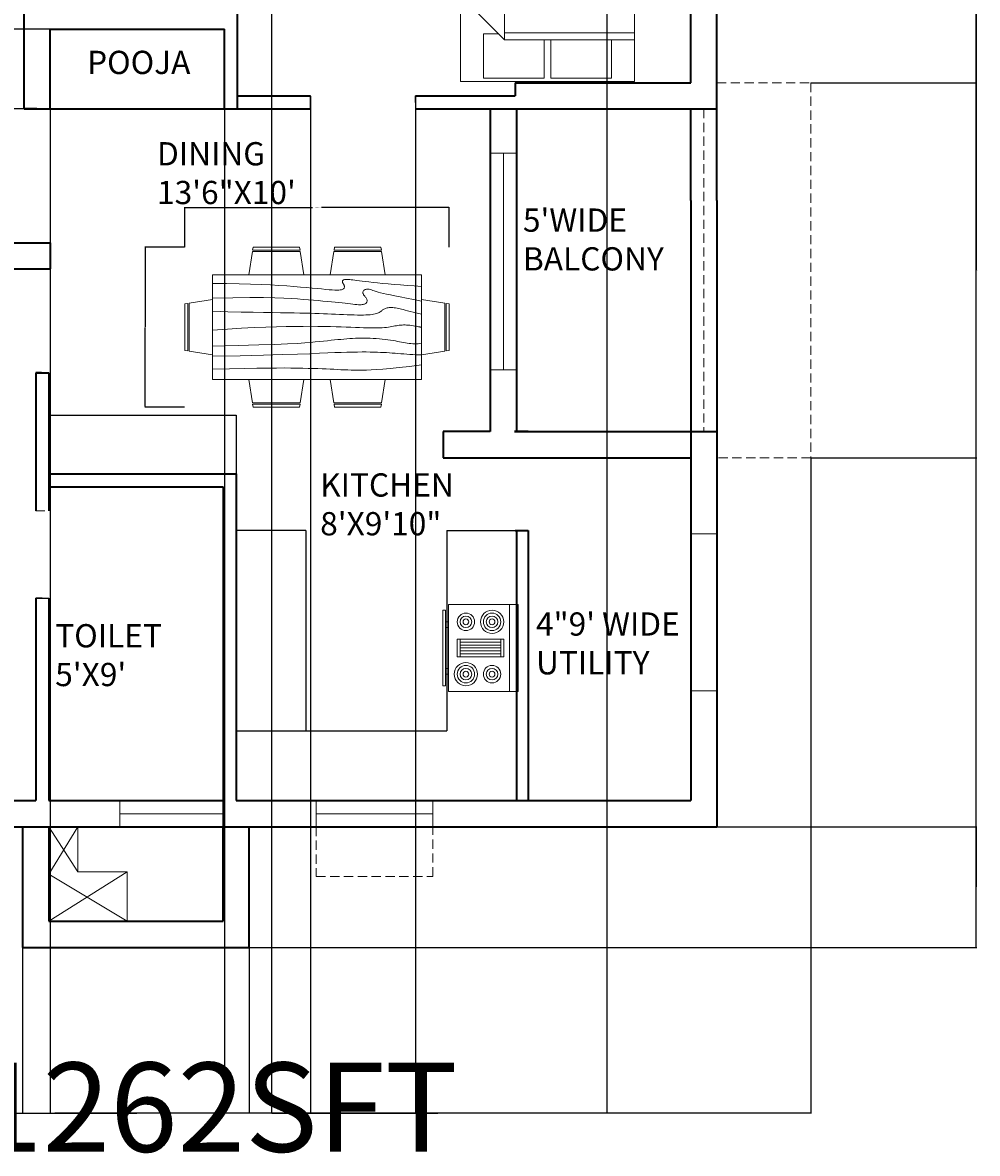
# Model space of a CAD drawing. Units: inches. Extents: x 276 to 912, y -567 to 621.
# Tile 3 of 7: x 583 to 912, y -567 to -178. Entities that reach past the tile are written whole.
import ezdxf

# ---------------------------------------------------------------- set-up
doc = ezdxf.new("R2010")
doc.units = ezdxf.units.IN
doc.linetypes.add('HIDDEN2', pattern=[4.7625, 3.175, -1.5875])
for name, color, linetype, lineweight in [('A-ANNO-DIMS', 2, 'Continuous', 18), ('A-ANNO-TEXT', 7, 'Continuous', 35), ('A-AREA-IDEN', 7, 'Continuous', 18), ('A-DOOR', 3, 'Continuous', 25), ('A-DOOR-HIDN', 3, 'HIDDEN2', 18), ('A-EQPM', 9, 'Continuous', 18), ('A-FLOR-CASE', 9, 'Continuous', 25), ('A-FLOR-OVHD', 8, 'HIDDEN2', 13), ('A-FLOR-SHFT', 8, 'Continuous', 18), ('A-FURN', 8, 'Continuous', 18), ('A-GLAZ', 4, 'Continuous', 18), ('A-WALL', 7, 'Continuous', 35), ('A-WALL-HIDN', 8, 'HIDDEN2', 18)]:
    doc.layers.add(name, color=color, linetype=linetype, lineweight=lineweight)
doc.dimstyles.get("Standard").update_dxf_attribs({"dimtxt": 0.18, "dimasz": 0.18, "dimexe": 0.18, "dimexo": 0.0625, "dimgap": 0.09, "dimtad": 0, "dimtih": 1, "dimtoh": 1, "dimdec": 4, "dimzin": 0, "dimdsep": 46, "dimtxsty": 'Standard', "dimcen": 0.09, "dimadec": 0, "dimazin": 0, "dimtfac": 1, "dimtdec": 4, "dimtofl": 0, "dimtmove": 0, "dimatfit": 3, "dimfxl": 1, "dimtolj": 1, "dimtzin": 0, "dimarcsym": 0})

# ---------------------------------------------------------------- blocks, each defined once
blk = doc.blocks.new('Dining Set - 36 x 72 in.')
for p, q in [((-22, 27.5), (-22.1562, 26.50042)), ((-22, 27.5), (-6, 27.5)), ((-5.8437, 26.49966), (-6, 27.5)), ((6, 27.5), (5.8438, 26.50042)), ((6, 27.5), (22, 27.5)), ((22.1563, 26.49966), (22, 27.5)), ((-22.2343, 26.00059), (-23.4847, 17.99762)), ((-22.2304, 26), (-5.7608, 26)), ((-5.8416, 26.5), (-22.1534, 26.5)), ((-4.5152, 17.99762), (-5.7655, 25.99926)), ((5.7657, 26.00059), (4.5153, 17.99762)), ((5.7696, 26), (22.2392, 26)), ((22.1584, 26.5), (5.8466, 26.5)), ((23.4848, 17.99762), (22.2345, 25.99926)), ((36, 18), (-36, 18)), ((-36, 18), (-36, -18)), ((36, -18), (36, 18)), ((-45.5, 8), (-44.5004, 8.15617)), ((-45.5, 8), (-45.5, -8)), ((-44.5, -8.15843), (-44.5, 8.15338)), ((-44.0006, 8.23428), (-35.9976, 9.48474)), ((-44, 8.23041), (-44, -8.23915)), ((44.0006, 8.23428), (35.9976, 9.48474)), ((44, 8.23041), (44, -8.23915)), ((44.5, -8.15843), (44.5, 8.15338)), ((45.5, 8), (44.5005, 8.15617)), ((45.5, 8), (45.5, -8)), ((-44.4997, -8.15631), (-45.5, -8)), ((-35.9976, -9.48476), (-43.9993, -8.2345)), ((35.9976, -9.48476), (43.9993, -8.2345)), ((44.4997, -8.15631), (45.5, -8)), ((-36, -18), (36, -18)), ((-22.2343, -26.0006), (-23.4847, -17.99762)), ((-4.5152, -17.99762), (-5.7655, -25.99928)), ((5.7657, -26.0006), (4.5153, -17.99762)), ((23.4848, -17.99762), (22.2345, -25.99928)), ((-22.2304, -26), (-5.7608, -26)), ((-22, -27.5), (-22.1562, -26.50044)), ((-5.8416, -26.5), (-22.1534, -26.5)), ((-5.8437, -26.49967), (-6, -27.5)), ((5.7696, -26), (22.2392, -26)), ((6, -27.5), (5.8438, -26.50044)), ((22.1584, -26.5), (5.8466, -26.5)), ((22.1563, -26.49967), (22, -27.5)), ((-22, -27.5), (-6, -27.5)), ((6, -27.5), (22, -27.5))]:
    blk.add_line(p, q)
for points in [[(-36, 15), (-31.1772, 14.97754), (-26.8079, 14.91406), (-22.8538, 14.81543), (-19.276, 14.6875), (-16.0362, 14.53613), (-13.0957, 14.36718), (-10.4159, 14.18652), (-7.9583, 14), (-5.6904, 13.81315), (-3.6035, 13.63021), (-1.6954, 13.45508), (0.0365, 13.29166), (1.5945, 13.14388), (2.9811, 13.01562), (4.1988, 12.9108), (5.25, 12.83333), (6.1393, 12.78613), (6.8802, 12.76823), (7.4883, 12.77767), (7.9792, 12.8125), (8.3685, 12.87077), (8.6719, 12.95052), (8.9049, 13.0498), (9.0833, 13.16666), (9.2205, 13.29899), (9.3216, 13.44401), (9.3895, 13.59879), (9.4271, 13.76041), (9.4373, 13.92594), (9.4232, 14.09245), (9.3875, 14.257), (9.3333, 14.41666), (9.2638, 14.56917), (9.1836, 14.71484), (9.0975, 14.85465), (9.0104, 14.98958), (8.9272, 15.1206), (8.8529, 15.2487), (8.7922, 15.37483), (8.75, 15.5), (8.7305, 15.62467), (8.7344, 15.74739), (8.7617, 15.86621), (8.8125, 15.97916), (8.8867, 16.08431), (8.9844, 16.17968), (9.1055, 16.26334), (9.25, 16.33333), (9.4189, 16.38802), (9.6172, 16.42708), (9.8506, 16.45052), (10.125, 16.45833), (10.4463, 16.45052), (10.8203, 16.42708), (11.2529, 16.38802), (11.75, 16.33333), (12.3184, 16.26318), (12.9694, 16.17838), (13.7151, 16.07991), (14.5677, 15.96875), (15.5395, 15.84586), (16.6426, 15.71224), (17.8893, 15.56884), (19.2917, 15.41666), (20.859, 15.25667), (22.5879, 15.08984), (24.4721, 14.91715), (26.5052, 14.73958), (28.6809, 14.5581), (30.9929, 14.3737), (33.4347, 14.18733), (36, 14)], [(-36, 10), (-28.9766, 10.14274), (-23.1725, 10.20442), (-18.4241, 10.19775), (-14.5677, 10.13541), (-11.4399, 10.03011), (-8.877, 9.89453), (-6.7154, 9.74137), (-4.7917, 9.58333), (-2.9698, 9.43082), (-1.2246, 9.28515), (0.4415, 9.14534), (2.026, 9.01041), (3.5266, 8.87939), (4.9408, 8.7513), (6.266, 8.62516), (7.5, 8.5), (8.6411, 8.37549), (9.6914, 8.2539), (10.6538, 8.13818), (11.5312, 8.03125), (12.3267, 7.93603), (13.043, 7.85547), (13.6831, 7.79248), (14.25, 7.75), (14.7471, 7.7303), (15.1797, 7.73307), (15.5537, 7.75732), (15.875, 7.80208), (16.1494, 7.86637), (16.3828, 7.94922), (16.5811, 8.04964), (16.75, 8.16666), (16.8944, 8.29915), (17.0143, 8.44531), (17.1089, 8.60319), (17.1771, 8.77083), (17.218, 8.94629), (17.2305, 9.1276), (17.2137, 9.31282), (17.1667, 9.5), (17.0895, 9.6875), (16.987, 9.875), (16.8649, 10.0625), (16.7292, 10.25), (16.5856, 10.4375), (16.4401, 10.625), (16.2985, 10.8125), (16.1667, 11), (16.05, 11.18733), (15.9518, 11.3737), (15.8752, 11.5581), (15.8229, 11.73958), (15.798, 11.91715), (15.8034, 12.08984), (15.842, 12.25667), (15.9167, 12.41666), (16.0295, 12.56836), (16.1784, 12.70833), (16.3605, 12.83268), (16.5729, 12.9375), (16.8127, 13.01888), (17.0768, 13.07291), (17.3625, 13.0957), (17.6667, 13.08333), (17.9894, 13.03312), (18.3418, 12.94726), (18.7382, 12.82918), (19.1927, 12.68229), (19.7195, 12.51001), (20.3327, 12.31575), (21.0465, 12.10294), (21.875, 11.875), (22.8357, 11.63354), (23.959, 11.37304), (25.2786, 11.08618), (26.8282, 10.76562), (28.6414, 10.40405), (30.752, 9.99414), (33.1936, 9.52856), (36, 9)], [(-36, 5.5), (-30.7157, 5.3348), (-26.069, 5.20963), (-21.9946, 5.11767), (-18.4271, 5.05208), (-15.3009, 5.00602), (-12.5508, 4.97265), (-10.1112, 4.94515), (-7.9167, 4.91666), (-5.909, 4.88167), (-4.0586, 4.83984), (-2.3429, 4.79215), (-0.7396, 4.73958), (0.7739, 4.6831), (2.22, 4.6237), (3.6213, 4.56233), (5, 4.5), (6.373, 4.43782), (7.7344, 4.3776), (9.0723, 4.32129), (10.375, 4.27083), (11.6309, 4.22819), (12.8281, 4.19531), (13.9551, 4.17415), (15, 4.16666), (15.954, 4.17448), (16.819, 4.19791), (17.6001, 4.23698), (18.3021, 4.29166), (18.9299, 4.36198), (19.4883, 4.44791), (19.9823, 4.54948), (20.4167, 4.66666), (20.7969, 4.79899), (21.1302, 4.94401), (21.4245, 5.09879), (21.6875, 5.26041), (21.9271, 5.42594), (22.1511, 5.59245), (22.3672, 5.757), (22.5834, 5.91666), (22.8065, 6.06868), (23.0404, 6.21093), (23.2879, 6.34147), (23.5521, 6.45833), (23.8358, 6.55957), (24.142, 6.64323), (24.4735, 6.70735), (24.8334, 6.75), (25.2235, 6.76969), (25.642, 6.76692), (26.0858, 6.74267), (26.5521, 6.69791), (27.0379, 6.63362), (27.5404, 6.55078), (28.0565, 6.45036), (28.5834, 6.33333), (29.1242, 6.19987), (29.7071, 6.04687), (30.3661, 5.87044), (31.1354, 5.66666), (32.0493, 5.43164), (33.142, 5.16146), (34.4475, 4.85221), (36, 4.5)], [(-36, -1), (-30.7915, -0.6591), (-26.0195, -0.38216), (-21.6519, -0.16284), (-17.6563, 0.00521), (-14.0005, 0.12833), (-10.6523, 0.21289), (-7.5796, 0.26522), (-4.75, 0.29166), (-2.134, 0.29793), (0.2878, 0.28711), (2.5317, 0.26163), (4.6146, 0.22396), (6.5529, 0.17651), (8.3633, 0.12174), (10.0623, 0.06209), (11.6667, 0), (13.1899, -0.06201), (14.6341, -0.1211), (15.9982, -0.17432), (17.2813, -0.21875), (18.4823, -0.25147), (19.6003, -0.26953), (20.6343, -0.27002), (21.5834, -0.25), (22.4481, -0.20768), (23.2357, -0.14584), (23.9549, -0.06836), (24.6146, 0.02083), (25.2235, 0.11784), (25.7904, 0.21875), (26.3241, 0.31966), (26.8334, 0.41666), (27.3265, 0.50618), (27.8099, 0.58593), (28.2894, 0.65397), (28.7709, 0.70833), (29.2601, 0.74707), (29.763, 0.76823), (30.2855, 0.76985), (30.8334, 0.75), (31.4088, 0.70784), (31.9994, 0.64713), (32.589, 0.57275), (33.1615, 0.48958), (33.7008, 0.4025), (34.1908, 0.3164), (34.6153, 0.23616), (34.9584, 0.16666), (35.2099, 0.11165), (35.3848, 0.07031), (35.504, 0.04069), (35.5886, 0.02083), (35.6594, 0.00879), (35.7377, 0.0026), (35.8442, 0.00032), (36, 0)], [(-36, -6.5), (-27.1843, -6.31267), (-20.084, -6.1263), (-14.469, -5.9419), (-10.1094, -5.76042), (-6.7752, -5.58285), (-4.2363, -5.41016), (-2.2629, -5.24333), (-0.625, -5.08334), (0.8708, -4.93099), (2.2715, -4.78646), (3.5872, -4.64974), (4.8281, -4.52084), (6.0046, -4.39974), (7.127, -4.28646), (8.2053, -4.18099), (9.25, -4.08334), (10.2705, -3.99382), (11.2734, -3.91407), (12.2647, -3.84603), (13.25, -3.79167), (14.2354, -3.75293), (15.2266, -3.73177), (16.2295, -3.73015), (17.25, -3.75), (18.2912, -3.79248), (19.3451, -3.85547), (20.4009, -3.93604), (21.4479, -4.03125), (22.4754, -4.13819), (23.4727, -4.25391), (24.4289, -4.37549), (25.3334, -4.5), (26.1785, -4.62492), (26.9694, -4.74935), (27.7145, -4.87281), (28.4219, -4.99479), (29.1, -5.11483), (29.7572, -5.23242), (30.4016, -5.34709), (31.0417, -5.45834), (31.6837, -5.56437), (32.3262, -5.65821), (32.9658, -5.73153), (33.599, -5.77604), (34.2224, -5.78345), (34.8327, -5.74545), (35.4264, -5.65373), (36, -5.5)], [(-36, -10), (-26.4022, -9.81299), (-18.4675, -9.62891), (-11.9839, -9.45069), (-6.7396, -9.28125), (-2.5226, -9.12354), (0.8789, -8.98047), (3.6769, -8.85498), (6.0833, -8.75), (8.2767, -8.66765), (10.3021, -8.60677), (12.1712, -8.56543), (13.8958, -8.54167), (15.4876, -8.53353), (16.9583, -8.53907), (18.3197, -8.55632), (19.5834, -8.58334), (20.7616, -8.61841), (21.8685, -8.66081), (22.9188, -8.71004), (23.9271, -8.76563), (24.9081, -8.82707), (25.8763, -8.89388), (26.8465, -8.96558), (27.8334, -9.04167), (28.8474, -9.12118), (29.8828, -9.20117), (30.93, -9.27824), (31.9792, -9.34896), (33.0205, -9.40991), (34.0443, -9.45768), (35.0407, -9.48885), (36, -9.5)], [(-36, -14.5), (-30.0881, -14.33513), (-25.0332, -14.21224), (-20.7312, -14.12647), (-17.0781, -14.07292), (-13.97, -14.04671), (-11.3027, -14.04297), (-8.9724, -14.05681), (-6.875, -14.08334), (-4.9224, -14.11833), (-3.0905, -14.16016), (-1.3709, -14.20785), (0.2448, -14.26042), (1.7647, -14.3169), (3.1973, -14.3763), (4.5507, -14.43767), (5.8333, -14.5), (7.0554, -14.5621), (8.235, -14.62175), (9.3922, -14.67652), (10.5469, -14.72396), (11.7192, -14.76164), (12.929, -14.78711), (14.1965, -14.79794), (15.5417, -14.79167), (16.9933, -14.76424), (18.6152, -14.70508), (20.4804, -14.60197), (22.6615, -14.44271), (25.2312, -14.21509), (28.2624, -13.9069), (31.8277, -13.50594), (36, -13)]]:
    blk.add_lwpolyline(points)
blk = doc.blocks.new('Bed - Queen')
for p, q in [((0, -80.00003), (0, 0)), ((0, 0), (59.99999, 0)), ((59.99999, 0), (59.99999, -80.00003)), ((7.99999, -1.2), (28.79998, -1.2)), ((7.99999, -14.4), (7.99999, -1.2)), ((28.79998, -1.2), (28.79998, -14.4)), ((31.19999, -1.2), (51.99999, -1.2)), ((31.19999, -14.4), (31.19999, -1.2)), ((51.99999, -1.2), (51.99999, -16.4)), ((0, -14.4), (44.8, -14.4)), ((59.99999, -29.6), (44.8, -14.4)), ((44.8, -14.4), (44.8, -29.6)), ((44.8, -16.8), (0, -16.8)), ((51.99999, -16.4), (46.79936, -16.4)), ((44.8, -29.6), (59.99999, -29.6)), ((59.99999, -80.00003), (0, -80.00003))]:
    blk.add_line(p, q)
blk = doc.blocks.new('Range-Oven - 30 in top')
for p, q in [((0, -3), (30, -3)), ((12, -6), (18, -6)), ((13, -20), (13, -6)), ((14, -6), (14, -20)), ((15, -20), (15, -6)), ((16, -6), (16, -20)), ((17, -20), (17, -6)), ((18, -20), (12, -20)), ((6, -24), (6, -25)), ((8, -25), (8, -24)), ((22, -25), (22, -24)), ((24, -24), (24, -25))]:
    blk.add_line(p, q)
for points in [[(0, -24), (0, 0), (30, 0), (30, -24)], [(12, -21), (12, -5), (18, -5), (18, -21)], [(2, -26), (2, -25), (28, -25), (28, -26)]]:
    blk.add_lwpolyline(points, close=True)
for centre, radius in [((6, -9), 4), ((6, -9), 3), ((6, -9), 2), ((24, -9), 3), ((24, -9), 2), ((6, -9), 1), ((24, -9), 1), ((6, -18), 3), ((24, -18), 4), ((24, -18), 3), ((6, -18), 2), ((6, -18), 1), ((24, -18), 2), ((24, -18), 1)]:
    blk.add_circle(centre, radius)
blk = doc.blocks.new('DOOR-JAMB-4.5IN')
for p, q in [((0, 2.25), (0, 4.5)), ((0, 4.5), (0, 0))]:
    blk.add_line(p, q)
blk = doc.blocks.new('*D18')
at = {"layer": 'A-ANNO-DIMS', "color": 0, "lineweight": -2, "transparency": 16777216}
for p, q in [((638.77, -255.04), (638.77, -241.28)), ((638.95, -241.46), (682.74, -241.46)), ((729.59, -241.46), (685.8, -241.46)), ((729.77, -255.04), (729.77, -241.28))]:
    blk.add_line(p, q, dxfattribs=at)
at = {"layer": 'A-ANNO-DIMS', "color": 0, "transparency": 16777216}
for points in [[(638.95, -241.43), (638.95, -241.49), (638.77, -241.46)], [(729.59, -241.43), (729.59, -241.49), (729.77, -241.46)]]:
    blk.add_solid(points, dxfattribs=at)
at = {"layer": 'Defpoints', "color": 0, "transparency": 16777216}
for p in [(729.77, -241.46), (638.77, -255.11), (729.77, -255.11)]:
    blk.add_point(p, dxfattribs=at)
at = {"layer": 'A-ANNO-DIMS', "color": 0, "transparency": 16777216, "insert": (684.27, -241.46), "char_height": 0.18, "attachment_point": 5}
blk.add_mtext('\\A1;DINING SET 91 TYP.', dxfattribs=at)
blk = doc.blocks.new('*D19')
at = {"layer": 'A-ANNO-DIMS', "color": 0, "lineweight": -2, "transparency": 16777216}
for p, q in [((638.7, -255.11), (624.94, -255.11)), ((625.12, -255.29), (625.12, -282.43)), ((625.12, -309.93), (625.12, -282.79)), ((638.7, -310.11), (624.94, -310.11))]:
    blk.add_line(p, q, dxfattribs=at)
at = {"layer": 'A-ANNO-DIMS', "color": 0, "transparency": 16777216}
for points in [[(625.09, -255.29), (625.15, -255.29), (625.12, -255.11)], [(625.09, -309.93), (625.15, -309.93), (625.12, -310.11)]]:
    blk.add_solid(points, dxfattribs=at)
at = {"layer": 'Defpoints', "color": 0, "transparency": 16777216}
for p in [(625.12, -255.11), (638.77, -255.11), (638.77, -310.11)]:
    blk.add_point(p, dxfattribs=at)
at = {"layer": 'A-ANNO-DIMS', "color": 0, "transparency": 16777216, "insert": (625.12, -282.61), "char_height": 0.18, "attachment_point": 5}
blk.add_mtext('\\A1;55 TYP.', dxfattribs=at)
blk = doc.blocks.new('*D24')
at = {"layer": 'A-ANNO-DIMS', "color": 0, "lineweight": -2, "transparency": 16777216}
for p, q in [((333.082179, 103.255751), (333.082179, -553.223061)), ((854.209085, -327.604004), (854.209085, -553.223061)), ((333.262179, -553.043061), (593.255632, -553.043061)), ((854.029085, -553.043061), (594.035632, -553.043061))]:
    blk.add_line(p, q, dxfattribs=at)
at = {"layer": 'A-ANNO-DIMS', "color": 0, "transparency": 16777216}
for points in [[(333.262179, -553.013061), (333.262179, -553.073061), (333.082179, -553.043061)], [(854.029085, -553.013061), (854.029085, -553.073061), (854.209085, -553.043061)]]:
    blk.add_solid(points, dxfattribs=at)
at = {"layer": 'Defpoints', "color": 0, "transparency": 16777216}
for p in [(333.082179, 103.318251), (854.209085, -327.541504), (854.209085, -553.043061)]:
    blk.add_point(p, dxfattribs=at)
at = {"layer": 'A-ANNO-DIMS', "color": 0, "transparency": 16777216, "insert": (593.645632, -553.043061), "char_height": 0.18, "attachment_point": 5}
blk.add_mtext('\\A1;521.1', dxfattribs=at)
blk = doc.blocks.new('*D25')
at = {"layer": 'A-ANNO-DIMS', "color": 0, "lineweight": -2, "transparency": 16777216}
for p, q in [((478.5, 564.29), (911.39, 564.29)), ((911.21, 564.11), (911.21, 34.31)), ((911.21, -495.86), (911.21, 33.95)), ((582.98, -496.04), (911.39, -496.04))]:
    blk.add_line(p, q, dxfattribs=at)
at = {"layer": 'A-ANNO-DIMS', "color": 0, "transparency": 16777216}
for points in [[(911.18, 564.11), (911.24, 564.11), (911.21, 564.29)], [(911.18, -495.86), (911.24, -495.86), (911.21, -496.04)]]:
    blk.add_solid(points, dxfattribs=at)
at = {"layer": 'Defpoints', "color": 0, "transparency": 16777216}
for p in [(478.44, 564.29), (582.92, -496.04), (911.21, -496.04)]:
    blk.add_point(p, dxfattribs=at)
at = {"layer": 'A-ANNO-DIMS', "color": 0, "transparency": 16777216, "insert": (911.21, 34.13), "char_height": 0.18, "attachment_point": 5}
blk.add_mtext('\\A1;1060.3', dxfattribs=at)
blk = doc.blocks.new('*D33')
at = {"layer": 'A-ANNO-DIMS', "color": 0, "lineweight": -2, "transparency": 16777216}
for p, q in [((553.582179, 65.246155), (553.582179, -553.223061)), ((668.582179, 65.246155), (668.582179, -553.223061)), ((553.762179, -553.043061), (610.812179, -553.043061)), ((668.402179, -553.043061), (611.352179, -553.043061))]:
    blk.add_line(p, q, dxfattribs=at)
at = {"layer": 'A-ANNO-DIMS', "color": 0, "transparency": 16777216}
for points in [[(553.762179, -553.013061), (553.762179, -553.073061), (553.582179, -553.043061)], [(668.402179, -553.013061), (668.402179, -553.073061), (668.582179, -553.043061)]]:
    blk.add_solid(points, dxfattribs=at)
at = {"layer": 'Defpoints', "color": 0, "transparency": 16777216}
for p in [(553.582179, 65.308655), (668.582179, 65.308655), (668.582179, -553.043061)]:
    blk.add_point(p, dxfattribs=at)
at = {"layer": 'A-ANNO-DIMS', "color": 0, "transparency": 16777216, "insert": (611.082179, -553.043061), "char_height": 0.18, "attachment_point": 5}
blk.add_mtext('\\A1;115', dxfattribs=at)
blk = doc.blocks.new('*D34')
at = {"layer": 'A-ANNO-DIMS', "color": 0, "lineweight": -2, "transparency": 16777216}
for p, q in [((668.58, 65.25), (668.58, -553.22)), ((784, 65.25), (784, -553.22)), ((668.76, -553.04), (725.81, -553.04)), ((783.82, -553.04), (726.77, -553.04))]:
    blk.add_line(p, q, dxfattribs=at)
at = {"layer": 'A-ANNO-DIMS', "color": 0, "transparency": 16777216}
for points in [[(668.76, -553.01), (668.76, -553.07), (668.58, -553.04)], [(783.82, -553.01), (783.82, -553.07), (784, -553.04)]]:
    blk.add_solid(points, dxfattribs=at)
at = {"layer": 'Defpoints', "color": 0, "transparency": 16777216}
for p in [(668.58, 65.31), (784, 65.31), (784, -553.04)]:
    blk.add_point(p, dxfattribs=at)
at = {"layer": 'A-ANNO-DIMS', "color": 0, "transparency": 16777216, "insert": (726.29, -553.04), "char_height": 0.18, "attachment_point": 5}
blk.add_mtext('\\A1;115.42', dxfattribs=at)
blk = doc.blocks.new('*D54')
at = {"layer": 'A-ANNO-DIMS', "color": 0, "lineweight": -2, "transparency": 16777216}
for p, q in [((821.980989, -64.541504), (911.389085, -64.541504)), ((911.209085, -64.721504), (911.209085, -259.361504)), ((911.209085, -454.361504), (911.209085, -259.721504)), ((821.980989, -454.541504), (911.389085, -454.541504))]:
    blk.add_line(p, q, dxfattribs=at)
at = {"layer": 'A-ANNO-DIMS', "color": 0, "transparency": 16777216}
for points in [[(911.179085, -64.721504), (911.239085, -64.721504), (911.209085, -64.541504)], [(911.179085, -454.361504), (911.239085, -454.361504), (911.209085, -454.541504)]]:
    blk.add_solid(points, dxfattribs=at)
at = {"layer": 'Defpoints', "color": 0, "transparency": 16777216}
for p in [(821.918489, -64.541504), (821.918489, -454.541504), (911.209085, -454.541504)]:
    blk.add_point(p, dxfattribs=at)
at = {"layer": 'A-ANNO-DIMS', "color": 0, "transparency": 16777216, "insert": (911.209085, -259.541504), "char_height": 0.18, "attachment_point": 5}
blk.add_mtext('\\A1;390', dxfattribs=at)
blk = doc.blocks.new('*D57')
at = {"layer": 'A-ANNO-DIMS', "color": 0, "lineweight": -2, "transparency": 16777216}
for p, q in [((582.918489, -496.105561), (582.918489, -553.223061)), ((660.918489, -496.105561), (660.918489, -553.223061)), ((583.098489, -553.043061), (621.678489, -553.043061)), ((660.738489, -553.043061), (622.158489, -553.043061))]:
    blk.add_line(p, q, dxfattribs=at)
at = {"layer": 'A-ANNO-DIMS', "color": 0, "transparency": 16777216}
for points in [[(583.098489, -553.013061), (583.098489, -553.073061), (582.918489, -553.043061)], [(660.738489, -553.013061), (660.738489, -553.073061), (660.918489, -553.043061)]]:
    blk.add_solid(points, dxfattribs=at)
at = {"layer": 'Defpoints', "color": 0, "transparency": 16777216}
for p in [(582.918489, -496.043061), (660.918489, -496.043061), (660.918489, -553.043061)]:
    blk.add_point(p, dxfattribs=at)
at = {"layer": 'A-ANNO-DIMS', "color": 0, "transparency": 16777216, "insert": (621.918489, -553.043061), "char_height": 0.18, "attachment_point": 5}
blk.add_mtext('\\A1;78', dxfattribs=at)
blk = doc.blocks.new('*D58')
at = {"layer": 'A-ANNO-DIMS', "color": 0, "lineweight": -2, "transparency": 16777216}
for p, q in [((660.98, -454.54), (911.39, -454.54)), ((911.21, -454.72), (911.21, -475.11)), ((911.21, -495.86), (911.21, -475.47)), ((660.98, -496.04), (911.39, -496.04))]:
    blk.add_line(p, q, dxfattribs=at)
at = {"layer": 'A-ANNO-DIMS', "color": 0, "transparency": 16777216}
for points in [[(911.18, -454.72), (911.24, -454.72), (911.21, -454.54)], [(911.18, -495.86), (911.24, -495.86), (911.21, -496.04)]]:
    blk.add_solid(points, dxfattribs=at)
at = {"layer": 'Defpoints', "color": 0, "transparency": 16777216}
for p in [(660.92, -454.54), (911.21, -454.54), (660.92, -496.04)]:
    blk.add_point(p, dxfattribs=at)
at = {"layer": 'A-ANNO-DIMS', "color": 0, "transparency": 16777216, "insert": (911.21, -475.29), "char_height": 0.18, "attachment_point": 5}
blk.add_mtext('\\A1;41.5', dxfattribs=at)
blk = doc.blocks.new('*D63')
at = {"layer": 'A-ANNO-DIMS', "color": 0, "lineweight": -2, "transparency": 16777216}
for p, q in [((682.059922, -203.068216), (682.059922, -553.223061)), ((718.16583, -207.568216), (718.16583, -553.223061)), ((682.239922, -553.043061), (699.617876, -553.043061)), ((717.98583, -553.043061), (700.607876, -553.043061))]:
    blk.add_line(p, q, dxfattribs=at)
at = {"layer": 'A-ANNO-DIMS', "color": 0, "transparency": 16777216}
for points in [[(682.239922, -553.013061), (682.239922, -553.073061), (682.059922, -553.043061)], [(717.98583, -553.013061), (717.98583, -553.073061), (718.16583, -553.043061)]]:
    blk.add_solid(points, dxfattribs=at)
at = {"layer": 'Defpoints', "color": 0, "transparency": 16777216}
for p in [(682.059922, -203.005716), (718.16583, -207.505716), (718.16583, -553.043061)]:
    blk.add_point(p, dxfattribs=at)
at = {"layer": 'A-ANNO-DIMS', "color": 0, "transparency": 16777216, "insert": (700.112876, -553.043061), "char_height": 0.18, "attachment_point": 5}
blk.add_mtext('\\A1;36.106', dxfattribs=at)
blk = doc.blocks.new('*D68')
at = {"layer": 'A-ANNO-DIMS', "color": 0, "lineweight": -2, "transparency": 16777216}
for p, q in [((592.418489, -207.568216), (592.418489, -553.223061)), ((652.418489, -207.568216), (652.418489, -553.223061)), ((592.598489, -553.043061), (622.193489, -553.043061)), ((652.238489, -553.043061), (622.643489, -553.043061))]:
    blk.add_line(p, q, dxfattribs=at)
at = {"layer": 'A-ANNO-DIMS', "color": 0, "transparency": 16777216}
for points in [[(592.598489, -553.013061), (592.598489, -553.073061), (592.418489, -553.043061)], [(652.238489, -553.013061), (652.238489, -553.073061), (652.418489, -553.043061)]]:
    blk.add_solid(points, dxfattribs=at)
at = {"layer": 'Defpoints', "color": 0, "transparency": 16777216}
for p in [(592.418489, -207.505716), (652.418489, -207.505716), (652.418489, -553.043061)]:
    blk.add_point(p, dxfattribs=at)
at = {"layer": 'A-ANNO-DIMS', "color": 0, "transparency": 16777216, "insert": (622.418489, -553.043061), "char_height": 0.18, "attachment_point": 5}
blk.add_mtext('\\A1;60', dxfattribs=at)
blk = doc.blocks.new('*D69')
at = {"layer": 'A-ANNO-DIMS', "color": 0, "lineweight": -2, "transparency": 16777216}
for p, q in [((592.355989, -180.041504), (275.902179, -180.041504)), ((276.082179, -180.221504), (276.082179, -193.59361)), ((276.082179, -207.325716), (276.082179, -193.95361)), ((592.355989, -207.505716), (275.902179, -207.505716))]:
    blk.add_line(p, q, dxfattribs=at)
at = {"layer": 'A-ANNO-DIMS', "color": 0, "transparency": 16777216}
for points in [[(276.052179, -180.221504), (276.112179, -180.221504), (276.082179, -180.041504)], [(276.052179, -207.325716), (276.112179, -207.325716), (276.082179, -207.505716)]]:
    blk.add_solid(points, dxfattribs=at)
at = {"layer": 'Defpoints', "color": 0, "transparency": 16777216}
for p in [(276.082179, -180.041504), (592.418489, -180.041504), (592.418489, -207.505716)]:
    blk.add_point(p, dxfattribs=at)
at = {"layer": 'A-ANNO-DIMS', "color": 0, "transparency": 16777216, "insert": (276.082179, -193.77361), "char_height": 0.18, "attachment_point": 5}
blk.add_mtext('\\A1;27.464', dxfattribs=at)
blk = doc.blocks.new('*D78')
at = {"layer": 'A-ANNO-DIMS', "color": 0, "lineweight": -2, "transparency": 16777216}
for p, q in [((854.271585, -198.505716), (911.389085, -198.505716)), ((911.209085, -198.685716), (911.209085, -262.84361)), ((911.209085, -327.361504), (911.209085, -263.20361)), ((854.271585, -327.541504), (911.389085, -327.541504))]:
    blk.add_line(p, q, dxfattribs=at)
at = {"layer": 'A-ANNO-DIMS', "color": 0, "transparency": 16777216}
for points in [[(911.179085, -198.685716), (911.239085, -198.685716), (911.209085, -198.505716)], [(911.179085, -327.361504), (911.239085, -327.361504), (911.209085, -327.541504)]]:
    blk.add_solid(points, dxfattribs=at)
at = {"layer": 'Defpoints', "color": 0, "transparency": 16777216}
for p in [(854.209085, -198.505716), (854.209085, -327.541504), (911.209085, -327.541504)]:
    blk.add_point(p, dxfattribs=at)
at = {"layer": 'A-ANNO-DIMS', "color": 0, "transparency": 16777216, "insert": (911.209085, -263.02361), "char_height": 0.18, "attachment_point": 5}
blk.add_mtext('\\A1;129.04', dxfattribs=at)

msp = doc.modelspace()

# ---------------------------------------------------------------- linework, layer by layer
at = {"layer": 'A-DOOR-HIDN'}
msp.add_line((587.4185, -345.8507), (591.9185, -345.8507), dxfattribs=at)
at = {"layer": 'A-FLOR-CASE'}
for p, q in [((591.9185, -312.8352), (656.4185, -312.8352)), ((656.4185, -312.8352), (656.4185, -333.0415)), ((680.4185, -352.5843), (656.4185, -352.5843)), ((680.4185, -352.5843), (680.4185, -421.5415)), ((728.9185, -352.5843), (728.9185, -421.5415)), ((728.9185, -352.5843), (752.4185, -352.5843)), ((656.4185, -421.5415), (728.9185, -421.5415))]:
    msp.add_line(p, q, dxfattribs=at)
at = {"layer": 'A-FLOR-OVHD'}
for p, q in [((821.9185, -198.5057), (854.2091, -198.5057)), ((854.2091, -198.5057), (854.2091, -327.5415)), ((854.2091, -327.5415), (821.9185, -327.5415)), ((684.0111, -454.5415), (684.0111, -471.6491)), ((724.1839, -471.6491), (724.1839, -454.5415)), ((684.0111, -471.6491), (724.1839, -471.6491))]:
    msp.add_line(p, q, dxfattribs=at)
at = {"layer": 'A-FLOR-SHFT'}
for p, q in [((591.9185, -470.7923), (601.9099, -454.5415)), ((591.9185, -454.5415), (601.9099, -470.0508)), ((601.9099, -470.0508), (601.9099, -454.5415)), ((591.9185, -487.0431), (618.9051, -470.0508)), ((618.9051, -487.0431), (591.9185, -470.7923)), ((618.9051, -470.0508), (601.9099, -470.0508)), ((618.9051, -487.0431), (618.9051, -470.0508))]:
    msp.add_line(p, q, dxfattribs=at)
at = {"layer": 'A-GLAZ'}
for p, q in [((752.9185, -222.7145), (743.9185, -222.7145)), ((743.9185, -222.7145), (748.4185, -222.7145)), ((748.4185, -222.7145), (748.4185, -297.3196)), ((748.4185, -297.3196), (743.9185, -297.3196)), ((743.9185, -297.3196), (752.9185, -297.3196)), ((812.9185, -353.7576), (821.9185, -353.7576)), ((821.9185, -353.7576), (821.9185, -407.7589)), ((821.9185, -407.7589), (812.9185, -407.7589)), ((616.4364, -445.5415), (616.4364, -454.5415)), ((684.0111, -445.5415), (684.0111, -454.5415)), ((724.1839, -450.0415), (724.1839, -445.5415)), ((724.1839, -445.5415), (724.1839, -454.5415)), ((616.4364, -454.5415), (616.4364, -450.0415)), ((616.4364, -450.0415), (651.9185, -450.0415)), ((684.0111, -454.5415), (684.0111, -450.0415)), ((684.0111, -450.0415), (724.1839, -450.0415))]:
    msp.add_line(p, q, dxfattribs=at)
at = {"layer": 'A-WALL'}
for p, q in [((821.9185, -238.9899), (821.9185, -64.5415)), ((583.4185, -207.5057), (583.4185, -73.5415)), ((656.9185, -207.5057), (656.9185, -73.5415)), ((812.9185, -198.5057), (812.9185, -73.5415)), ((592.4185, -207.5057), (592.4185, -180.0415)), ((592.4185, -180.0415), (652.4185, -180.0415)), ((652.4185, -207.5057), (652.4185, -180.0415)), ((752.4806, -198.5057), (812.9185, -198.5057)), ((752.4806, -198.5057), (752.4806, -203.0057)), ((656.9185, -203.0057), (682.0599, -203.0057)), ((718.1658, -203.0057), (752.4806, -203.0057)), ((587.8199, -207.5057), (583.4185, -207.5057)), ((583.4185, -207.5057), (592.4185, -207.5057)), ((592.4185, -207.5057), (656.9185, -207.5057)), ((656.9185, -207.5057), (682.0599, -207.5057)), ((718.1658, -207.5057), (812.9185, -207.5057)), ((743.9185, -207.5057), (743.9185, -318.5415)), ((752.9185, -207.5057), (752.9185, -318.5415)), ((812.9185, -238.9899), (812.9185, -207.5057)), ((812.9185, -207.5057), (821.9185, -207.5057)), ((812.9185, -238.9899), (812.9185, -445.5415)), ((821.9185, -238.9899), (821.9185, -454.5415)), ((457.4185, -253.5415), (592.4185, -253.5415)), ((592.4185, -253.5415), (592.4185, -262.5415)), ((457.4185, -262.5415), (592.4185, -262.5415)), ((587.4185, -298.3217), (587.4185, -345.8507)), ((589.402, -298.3217), (587.4185, -298.3217)), ((587.4185, -298.3217), (591.9185, -298.3217)), ((591.9185, -298.3217), (591.9185, -345.8507)), ((743.9185, -318.5415), (727.7175, -318.5415)), ((727.7175, -318.5415), (727.7175, -327.5415)), ((756.9185, -318.5415), (752.2534, -318.5415)), ((752.2534, -318.5415), (812.9185, -318.5415)), ((812.9185, -318.5415), (821.9185, -318.5415)), ((727.7175, -327.5415), (752.4185, -327.5415)), ((752.4185, -327.5415), (812.9185, -327.5415)), ((591.9185, -333.0415), (656.4185, -333.0415)), ((656.4185, -333.0415), (656.4185, -445.5415)), ((591.9185, -337.5415), (651.9185, -337.5415)), ((651.9185, -337.5415), (651.9185, -454.5415)), ((752.4185, -352.5843), (756.9185, -352.5843)), ((752.9185, -352.5843), (752.9185, -445.5415)), ((756.9185, -352.5843), (756.9185, -445.5415)), ((587.4185, -375.8611), (587.4185, -445.5415)), ((591.9185, -375.8611), (591.9185, -445.5415)), ((457.4185, -445.5415), (587.4185, -445.5415)), ((591.9185, -445.5415), (651.9185, -445.5415)), ((656.4185, -445.5415), (812.9185, -445.5415)), ((457.4185, -454.5415), (812.9185, -454.5415)), ((582.9185, -454.5415), (582.9185, -496.0431)), ((591.9185, -454.5415), (591.9185, -487.0431)), ((651.9185, -487.0431), (651.9185, -454.5415)), ((660.9185, -496.0431), (660.9185, -454.5415)), ((812.9185, -454.5415), (821.9185, -454.5415)), ((591.9185, -487.0431), (651.9185, -487.0431)), ((582.9185, -496.0431), (660.9185, -496.0431))]:
    msp.add_line(p, q, dxfattribs=at)
at = {"layer": 'A-WALL-HIDN'}
msp.add_line((817.4185, -207.5057), (817.4185, -318.5415), dxfattribs=at)

# ---------------------------------------------------------------- block references
at = {"layer": 'A-DOOR'}
for p, rotation in [((682.06, -203.0055), 180), ((591.9187, -375.8611), 90)]:
    msp.add_blockref('DOOR-JAMB-4.5IN', p, dxfattribs=dict(at, rotation=rotation))
msp.add_blockref('DOOR-JAMB-4.5IN', (718.1658, -207.506), dxfattribs=at)
at = {"layer": 'A-EQPM', "rotation": 270}
msp.add_blockref('Range-Oven - 30 in top', (753.5155, -378.0102), dxfattribs=at)
at = {"layer": 'A-FURN', "rotation": 180}
msp.add_blockref('Bed - Queen', (793.6066, -198.0637), dxfattribs=at)
at = {"layer": 'A-FURN'}
msp.add_blockref('Dining Set - 36 x 72 in.', (684.2673, -282.6069), dxfattribs=at)

# ---------------------------------------------------------------- texts
at = {"layer": 'A-ANNO-TEXT', "insert": (566.519, -535.6866), "char_height": 30.703761, "attachment_point": 1}
msp.add_mtext_dynamic_manual_height_columns('{\\fTimes New Roman|b0|i0|c0|p18;1262SFT}', width=239.005817, gutter_width=47.9746, heights=[0], dxfattribs=at)
at = {"layer": 'A-AREA-IDEN', "char_height": 8, "attachment_point": 1}
for s, insert in [('{\\fTimes New Roman|b0|i0|c0|p18;POOJA}', (605.1011, -187.4871)), ('{\\fTimes New Roman|b0|i0|c0|p18;DINING\\P13\'6"X10\'}', (629.1892, -218.9224)), ("{\\fTimes New Roman|b0|i0|c0|p18;5'WIDE BALCONY}", (755.1445, -241.7568)), ('{\\fTimes New Roman|b0|i0|c0|p18;KITCHEN\\P8\'X9\'10"}', (685.3482, -332.9075)), ('{\\fTimes New Roman|b0|i0|c0|p18;4"9\' WIDE UTILITY}', (759.6445, -380.7582)), ("{\\fTimes New Roman|b0|i0|c0|p18;TOILET\\P5'X9'}", (594.1445, -384.8008))]:
    msp.add_mtext_dynamic_manual_height_columns(s, width=62.274017, gutter_width=12.5, heights=[0], dxfattribs=dict(at, insert=insert))

# ---------------------------------------------------------------- dimensions: what is measured, and where the dimension line sits
at = {"layer": 'A-ANNO-DIMS'}
for base, p1, p2, override, picture, middle in [((911.2091, -496.0431), (478.4357, 564.2937), (582.9185, -496.0431), {"dimdec": 1, "dimlfac": 1, "dimrnd": 0, "dimzin": 0, "dimdsep": 46, "dimlunit": 2}, '*D25', (911.2091, 34.1253)), ((911.2091, -454.5415), (821.9185, -64.5415), (821.9185, -454.5415), {"dimdec": 0, "dimlfac": 1, "dimrnd": 0, "dimzin": 0, "dimdsep": 46, "dimlunit": 2}, '*D54', (911.2091, -259.5415)), ((276.0822, -180.0415), (592.4185, -207.5057), (592.4185, -180.0415), {"dimdec": 3, "dimlfac": 1, "dimrnd": 0, "dimzin": 0, "dimdsep": 46, "dimlunit": 2}, '*D69', (276.0822, -193.7736)), ((911.2091, -327.5415), (854.2091, -198.5057), (854.2091, -327.5415), {"dimdec": 2, "dimlfac": 1, "dimrnd": 0, "dimzin": 0, "dimdsep": 46, "dimlunit": 2}, '*D78', (911.2091, -263.0236)), ((911.2091, -454.5415), (660.9185, -496.0431), (660.9185, -454.5415), {"dimdec": 1, "dimlfac": 1, "dimrnd": 0, "dimzin": 0, "dimdsep": 46, "dimlunit": 2}, '*D58', (911.2091, -475.2923))]:
    dim = msp.add_linear_dim(base=base, p1=p1, p2=p2, angle=90, dimstyle='Standard', override=override, dxfattribs=at)
    dim.commit()
    dim.dimension.update_dxf_attribs({"geometry": picture, "text_midpoint": middle})
for base, p1, p2, override, picture, middle in [((854.2091, -553.0431), (333.0822, 103.3183), (854.2091, -327.5415), {"dimdec": 1, "dimlfac": 1, "dimrnd": 0, "dimzin": 0, "dimdsep": 46, "dimlunit": 2}, '*D24', (593.6456, -553.0431)), ((668.5822, -553.0431), (553.5822, 65.3087), (668.5822, 65.3087), {"dimdec": 0, "dimlfac": 1, "dimrnd": 0, "dimzin": 0, "dimdsep": 46, "dimlunit": 2}, '*D33', (611.0822, -553.0431)), ((783.9998, -553.0431), (668.5822, 65.3087), (783.9998, 65.3087), {"dimdec": 2, "dimlfac": 1, "dimrnd": 0, "dimzin": 0, "dimdsep": 46, "dimlunit": 2}, '*D34', (726.291, -553.0431)), ((718.1658, -553.0431), (682.0599, -203.0057), (718.1658, -207.5057), {"dimdec": 3, "dimlfac": 1, "dimrnd": 0, "dimzin": 0, "dimdsep": 46, "dimlunit": 2}, '*D63', (700.1129, -553.0431)), ((652.4185, -553.0431), (592.4185, -207.5057), (652.4185, -207.5057), {"dimdec": 0, "dimlfac": 1, "dimrnd": 0, "dimzin": 0, "dimdsep": 46, "dimlunit": 2}, '*D68', (622.4185, -553.0431)), ((660.9185, -553.0431), (582.9185, -496.0431), (660.9185, -496.0431), {"dimdec": 0, "dimlfac": 1, "dimrnd": 0, "dimzin": 0, "dimdsep": 46, "dimlunit": 2}, '*D57', (621.9185, -553.0431))]:
    dim = msp.add_linear_dim(base=base, p1=p1, p2=p2, dimstyle='Standard', override=override, dxfattribs=at)
    dim.commit()
    dim.dimension.update_dxf_attribs({"geometry": picture, "text_midpoint": middle})
dim = msp.add_linear_dim(base=(729.7673, -241.4569), p1=(638.7673, -255.1069), p2=(729.7673, -255.1069), text='DINING SET <> TYP.', dimstyle='Standard', override={"dimdec": 0, "dimlfac": 1, "dimrnd": 0, "dimzin": 0, "dimdsep": 46, "dimlunit": 2}, dxfattribs=at)
dim.commit()
dim.dimension.update_dxf_attribs({"geometry": '*D18', "text_midpoint": (684.2673, -241.4569)})
dim = msp.add_linear_dim(base=(625.1173, -255.1069), p1=(638.7673, -310.1069), p2=(638.7673, -255.1069), angle=90, text='<> TYP.', dimstyle='Standard', override={"dimdec": 0, "dimlfac": 1, "dimrnd": 0, "dimzin": 0, "dimdsep": 46, "dimlunit": 2}, dxfattribs=at)
dim.commit()
dim.dimension.update_dxf_attribs({"geometry": '*D19', "text_midpoint": (625.1173, -282.6069)})

doc.saveas('drawing.dxf')
